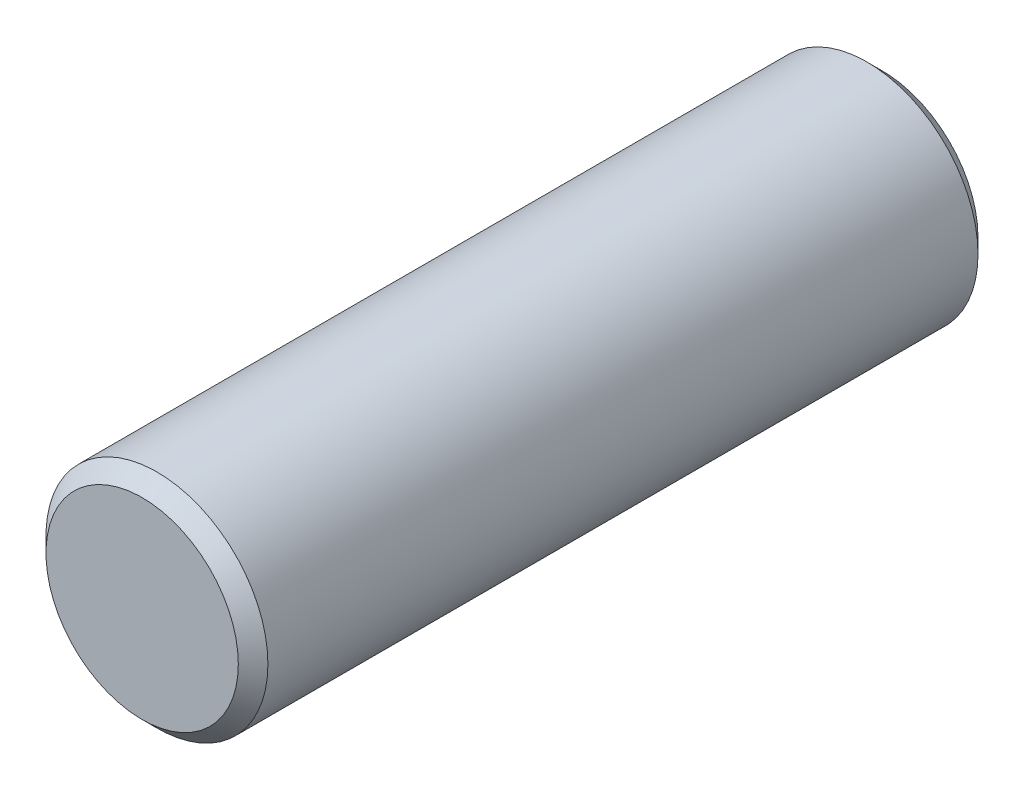
from build123d import *

# Parameters (mm, degrees)
PIN_PROFILE_3_R          = 1.5
PIN_BODY_3X10_DEPTH      = 5
END_CHAMFERS_0_2X45_SIZE = 0.2


with BuildPart() as part:
    # Pin Profile Ø3 → Pin Body Ø3x10 (new, symmetric)
    with BuildSketch(Plane.XY):
        Circle(PIN_PROFILE_3_R)
    extrude(amount=PIN_BODY_3X10_DEPTH, both=True)

    # End Chamfers 0.2x45°
    end_chamfers_0_2x45_edges = [part.edges().sort_by_distance(p)[0] for p in [
        (-1.5, 0, -5),
        (-1.5, 0, 5),
    ]]
    chamfer(end_chamfers_0_2x45_edges, length=END_CHAMFERS_0_2X45_SIZE)


solid = part.part
